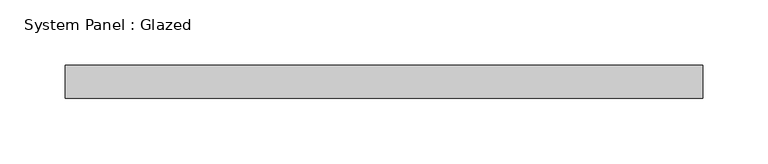
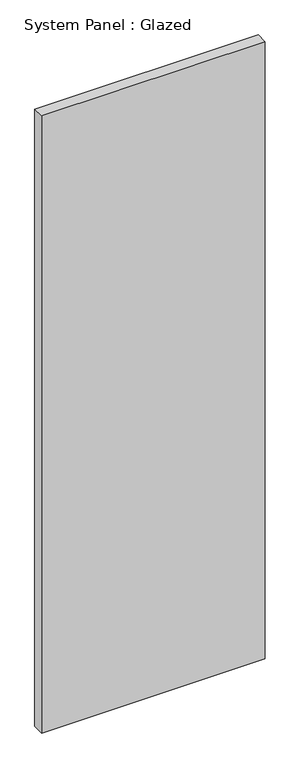
"""IFC4 building model written with IfcOpenShell, lengths in millimetres: plate geometry, System Panel : Glazed."""

from ifc_helpers import new_model, si_unit, origin, origin_with_axes, place, context, project, spatial, polyline, outline, extrude, source, transform, mapped, element, save


def system_panel_glazed_b96e00cd(model_context):
    return source(origin(), model_context, "Body", "SweptSolid", [
        extrude(outline(polyline([(244.475, 19.05), (-244.475, 19.05), (-244.475, 44.45), (244.475, 44.45), (244.475, 19.05)])), origin_with_axes(), (0.0, 0.0, 1.0), 1426.5106693),
    ])


if __name__ == "__main__":
    model = new_model("IFC4")
    model_context = context("Model", 3, world=origin())
    ifc_project = project(units=[si_unit("LENGTHUNIT", "METRE", prefix="MILLI")], contexts=[model_context])
    site = spatial("IfcSite", under=ifc_project)
    building = spatial("IfcBuilding", under=site)
    placement = place(None, origin())
    system_panel_glazed_shape = system_panel_glazed_b96e00cd(model_context)
    element("IfcPlate", 1, ObjectType="System Panel : Glazed", at=placement, inside=building, context=model_context, shape_type="MappedRepresentation", body=[
        mapped(system_panel_glazed_shape, transform((0.0, 0.0, 0.0), x_axis=(1.0, 0.0, 0.0), y_axis=(0.0, 1.0, 0.0), z_axis=(0.0, 0.0, 1.0))),
    ])
    save(model, "model.ifc")

# Revit data of these elements
# Type "System Panel : Glazed"
#   Construction Type Id = "GSP4R"
#   Analytic Construction = "1/8 in Pilkington single glazing"
#   Visual Light Transmittance = 0.9
#   Solar Heat Gain Coefficient = 0.86
#   Heat Transfer Coefficient (U) = 1.18115 BTU/(h·ft²·°F)
#   Define Thermal Properties by = 1
# Element 1 (IfcPlate, "System Panel : Glazed")
#   Materials on its faces: "Glass"
# Materials
#   "Glass": class "Glass", colour RGB 0 128 192, transparency 0.75, Description = "Soda Lime Glass", Cost = 0
